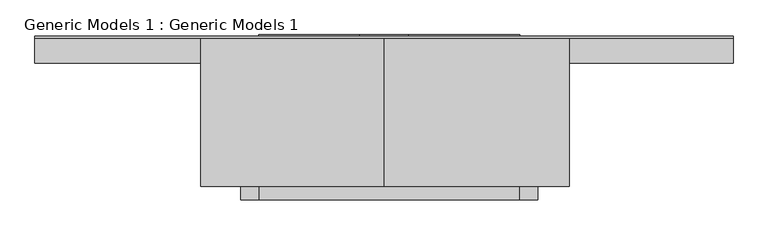
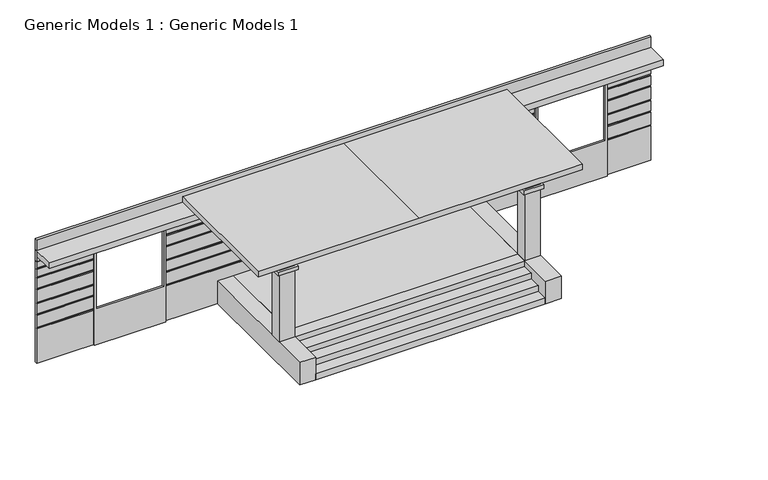
"""IFC4 building model written with IfcOpenShell, lengths in millimetres: proxy geometry, Generic Models 1 : Generic Models 1."""

from ifc_helpers import new_model, si_unit, frame, origin, origin_with_axes, place, context, project, spatial, polyline, outline, extrude, faceted_brep, source, transform, mapped, element, save


def generic_models_1_generic_models_1_130779d0(model_context):
    return source(origin(), model_context, "Body", "SolidModel", [
        extrude(outline(polyline([(2743.2, 5799.8347658), (2743.2, 3971.0347658), (0.0, 3971.0347658), (0.0, 5799.8347658), (2743.2, 5799.8347658)]), holes=[polyline([(2679.7, 5736.3347658), (977.9, 5736.3347658), (977.9, 4034.5347658), (2679.7, 4034.5347658), (2679.7, 5736.3347658)])]), frame((0.0, -1778.7594336, 0.0), z_axis=(0.0, 1.0, 0.0), x_axis=(0.0, 0.0, 1.0)), (0.0, 0.0, 1.0), 50.8),
        extrude(outline(polyline([(2743.2, -5477.7652342), (2743.2, -7306.5652342), (0.0, -7306.5652342), (0.0, -5477.7652342), (2743.2, -5477.7652342)]), holes=[polyline([(2679.7, -5541.2652342), (977.9, -5541.2652342), (977.9, -7243.0652342), (2679.7, -7243.0652342), (2679.7, -5541.2652342)])]), frame((0.0, -1778.7594336, 0.0), z_axis=(0.0, 1.0, 0.0), x_axis=(0.0, 0.0, 1.0)), (0.0, 0.0, 1.0), 50.8),
        extrude(outline(polyline([(-4131.5652342, -4452.9371224), (-4131.5652342, -4148.1371224), (-3725.1652342, -4148.1371224), (-3725.1652342, -4452.9371224), (-4131.5652342, -4452.9371224)])), frame((0.0, 0.0, 2540.0), z_axis=(0.0, 0.0, 1.0), x_axis=(1.0, 0.0, 0.0)), (0.0, 0.0, 1.0), 508.0),
        extrude(outline(polyline([(2142.2347658, -4452.9371224), (2142.2347658, -4148.1371224), (2548.6347658, -4148.1371224), (2548.6347658, -4452.9371224), (2142.2347658, -4452.9371224)])), frame((0.0, 0.0, 2540.0), z_axis=(0.0, 0.0, 1.0), x_axis=(1.0, 0.0, 0.0)), (0.0, 0.0, 1.0), 508.0),
        extrude(outline(polyline([(2599.4347658, -4503.7371224), (2091.4347658, -4503.7371224), (2091.4347658, -4097.3371224), (2599.4347658, -4097.3371224), (2599.4347658, -4503.7371224)])), frame((0.0, 0.0, 2438.4), z_axis=(0.0, 0.0, 1.0), x_axis=(1.0, 0.0, 0.0)), (0.0, 0.0, 1.0), 101.6),
        extrude(outline(polyline([(-3674.3652342, -4503.7371224), (-4182.3652342, -4503.7371224), (-4182.3652342, -4097.3371224), (-3674.3652342, -4097.3371224), (-3674.3652342, -4503.7371224)])), frame((0.0, 0.0, 2438.4), z_axis=(0.0, 0.0, 1.0), x_axis=(1.0, 0.0, 0.0)), (0.0, 0.0, 1.0), 101.6),
        extrude(outline(polyline([(2548.6347658, -4452.9371224), (2142.2347658, -4452.9371224), (2142.2347658, -4148.1371224), (2548.6347658, -4148.1371224), (2548.6347658, -4452.9371224)])), frame((0.0, 0.0, 609.6), z_axis=(0.0, 0.0, 1.0), x_axis=(1.0, 0.0, 0.0)), (0.0, 0.0, 1.0), 1828.8),
        extrude(outline(polyline([(-4131.5652342, -4148.1371224), (-3725.1652342, -4148.1371224), (-3725.1652342, -4452.9371224), (-4131.5652342, -4452.9371224), (-4131.5652342, -4148.1371224)])), frame((0.0, 0.0, 609.6), z_axis=(0.0, 0.0, 1.0), x_axis=(1.0, 0.0, 0.0)), (0.0, 0.0, 1.0), 1828.8),
        extrude(outline(polyline([(3048.0, -905.7652342), (3048.0, 3259.8347658), (3200.4, 3259.8347658), (3200.4, -905.7652342), (3200.4, -5020.5652342), (3048.0, -5020.5652342), (3048.0, -905.7652342)])), frame((0.0, -5062.5371224, 0.0), z_axis=(0.0, 1.0, 0.0), x_axis=(0.0, 0.0, 1.0)), (0.0, 0.0, 1.0), 3334.5776888),
        extrude(outline(polyline([(6942.8347658, -1727.9594336), (-8754.3652342, -1727.9594336), (-8754.3652342, -1677.1594336), (6942.8347658, -1677.1594336), (6942.8347658, -1727.9594336)])), frame((0.0, 0.0, 2743.2), z_axis=(0.0, 0.0, 1.0), x_axis=(1.0, 0.0, 0.0)), (0.0, 0.0, 1.0), 595.6731526),
        faceted_brep([(-8754.3652342, -1727.9594336, 0.0), (-4131.5652342, -1727.9594336, 0.0), (-4131.5652342, -1727.9594336, 600.1351718), (-1464.5652342, -1727.9594336, 600.1351718), (-1464.5652342, -1727.9594336, 2743.2), (-1997.9652342, -1727.9594336, 2743.2), (-1997.9652342, -1727.9594336, 1066.8), (-3521.9652342, -1727.9594336, 1066.8), (-3521.9652342, -1727.9594336, 1295.4), (-5477.7652342, -1727.9594336, 1295.4), (-5477.7652342, -1727.9594336, 969.0865476), (-3211.4976527, -1727.9594336, 969.0865476), (-1489.9652342, -1727.9594336, 969.0865476), (-1489.9652342, -1727.9594336, 926.1227307), (-3217.0111175, -1727.9594336, 926.1227307), (-5477.7652342, -1727.9594336, 926.1227307), (-5477.7652342, -1727.9594336, 914.4), (-7306.5652342, -1727.9594336, 914.4), (-7306.5652342, -1727.9594336, 926.1227307), (-8754.3652342, -1727.9594336, 926.1227307), (-1972.5652342, -1727.9594336, 1338.363817), (-1489.9652342, -1727.9594336, 1338.363817), (-1489.9652342, -1727.9594336, 1295.4), (-1972.5652342, -1727.9594336, 1295.4), (-1972.5652342, -1727.9594336, 1643.163817), (-1489.9652342, -1727.9594336, 1643.163817), (-1489.9652342, -1727.9594336, 1600.2), (-1972.5652342, -1727.9594336, 1600.2), (-1972.5652342, -1727.9594336, 2024.163817), (-1489.9652342, -1727.9594336, 2024.163817), (-1489.9652342, -1727.9594336, 1981.2), (-1972.5652342, -1727.9594336, 1981.2), (-1972.5652342, -1727.9594336, 2328.963817), (-1489.9652342, -1727.9594336, 2328.963817), (-1489.9652342, -1727.9594336, 2286.0), (-1972.5652342, -1727.9594336, 2286.0), (-1972.5652342, -1727.9594336, 2582.963817), (-1489.9652342, -1727.9594336, 2582.963817), (-1489.9652342, -1727.9594336, 2540.0), (-1972.5652342, -1727.9594336, 2540.0), (-3521.9652342, -1727.9594336, 2743.2), (-5477.7652342, -1727.9594336, 2743.2), (-5477.7652342, -1727.9594336, 2582.963817), (-3521.9652342, -1727.9594336, 2582.963817), (-7306.5652342, -1727.9594336, 2743.2), (-8754.3652342, -1727.9594336, 2743.2), (-8754.3652342, -1727.9594336, 2582.963817), (-7306.5652342, -1727.9594336, 2582.963817), (-8754.3652342, -1727.9594336, 1295.4), (-8754.3652342, -1727.9594336, 969.0865476), (-7306.5652342, -1727.9594336, 969.0865476), (-7306.5652342, -1727.9594336, 1295.4), (-8754.3652342, -1727.9594336, 1600.2), (-8754.3652342, -1727.9594336, 1338.363817), (-7306.5652342, -1727.9594336, 1338.363817), (-7306.5652342, -1727.9594336, 1600.2), (-8754.3652342, -1727.9594336, 1981.2), (-8754.3652342, -1727.9594336, 1643.163817), (-7306.5652342, -1727.9594336, 1643.163817), (-7306.5652342, -1727.9594336, 1981.2), (-8754.3652342, -1727.9594336, 2286.0), (-8754.3652342, -1727.9594336, 2024.163817), (-7306.5652342, -1727.9594336, 2024.163817), (-7306.5652342, -1727.9594336, 2286.0), (-8754.3652342, -1727.9594336, 2540.0), (-8754.3652342, -1727.9594336, 2328.963817), (-7306.5652342, -1727.9594336, 2328.963817), (-7306.5652342, -1727.9594336, 2540.0), (-3521.9652342, -1727.9594336, 1338.363817), (-3521.9652342, -1727.9594336, 1600.2), (-5477.7652342, -1727.9594336, 1600.2), (-5477.7652342, -1727.9594336, 1338.363817), (-3521.9652342, -1727.9594336, 1643.163817), (-3521.9652342, -1727.9594336, 1981.2), (-5477.7652342, -1727.9594336, 1981.2), (-5477.7652342, -1727.9594336, 1643.163817), (-3521.9652342, -1727.9594336, 2024.163817), (-3521.9652342, -1727.9594336, 2286.0), (-5477.7652342, -1727.9594336, 2286.0), (-5477.7652342, -1727.9594336, 2024.163817), (-3521.9652342, -1727.9594336, 2328.963817), (-3521.9652342, -1727.9594336, 2540.0), (-5477.7652342, -1727.9594336, 2540.0), (-5477.7652342, -1727.9594336, 2328.963817), (-4131.5652342, -1677.1594336, 600.1351718), (-4131.5652342, -1677.1594336, 0.0), (-8754.3652342, -1677.1594336, 0.0), (-8754.3652342, -1677.1594336, 2743.2), (-7306.5652342, -1677.1594336, 2743.2), (-7306.5652342, -1677.1594336, 914.4), (-5477.7652342, -1677.1594336, 914.4), (-5477.7652342, -1677.1594336, 2743.2), (-3521.9652342, -1677.1594336, 2743.2), (-3521.9652342, -1677.1594336, 1066.8), (-1997.9652342, -1677.1594336, 1066.8), (-1997.9652342, -1677.1594336, 2743.2), (-1464.5652342, -1677.1594336, 2743.2), (-1464.5652342, -1677.1594336, 600.1351718), (-8754.3652342, -1702.5594336, 926.1227307), (-8754.3652342, -1702.5594336, 969.0865476), (-8754.3652342, -1702.5594336, 1295.4), (-8754.3652342, -1702.5594336, 1338.363817), (-8754.3652342, -1702.5594336, 1600.2), (-8754.3652342, -1702.5594336, 1643.163817), (-8754.3652342, -1702.5594336, 1981.2), (-8754.3652342, -1702.5594336, 2024.163817), (-8754.3652342, -1702.5594336, 2286.0), (-8754.3652342, -1702.5594336, 2328.963817), (-8754.3652342, -1702.5594336, 2540.0), (-8754.3652342, -1702.5594336, 2582.963817), (-5477.7652342, -1702.5594336, 926.1227307), (-5477.7652342, -1702.5594336, 969.0865476), (-5477.7652342, -1702.5594336, 1295.4), (-5477.7652342, -1702.5594336, 1338.363817), (-5477.7652342, -1702.5594336, 1600.2), (-5477.7652342, -1702.5594336, 1643.163817), (-5477.7652342, -1702.5594336, 1981.2), (-5477.7652342, -1702.5594336, 2024.163817), (-5477.7652342, -1702.5594336, 2286.0), (-5477.7652342, -1702.5594336, 2328.963817), (-5477.7652342, -1702.5594336, 2540.0), (-5477.7652342, -1702.5594336, 2582.963817), (-7306.5652342, -1702.5594336, 2582.963817), (-7306.5652342, -1702.5594336, 2540.0), (-7306.5652342, -1702.5594336, 2328.963817), (-7306.5652342, -1702.5594336, 2286.0), (-7306.5652342, -1702.5594336, 2024.163817), (-7306.5652342, -1702.5594336, 1981.2), (-7306.5652342, -1702.5594336, 1643.163817), (-7306.5652342, -1702.5594336, 1600.2), (-7306.5652342, -1702.5594336, 1338.363817), (-7306.5652342, -1702.5594336, 1295.4), (-7306.5652342, -1702.5594336, 969.0865476), (-7306.5652342, -1702.5594336, 926.1227307), (-3521.9652342, -1702.5594336, 2582.963817), (-3521.9652342, -1702.5594336, 2540.0), (-3521.9652342, -1702.5594336, 2328.963817), (-3521.9652342, -1702.5594336, 2286.0), (-3521.9652342, -1702.5594336, 2024.163817), (-3521.9652342, -1702.5594336, 1981.2), (-3521.9652342, -1702.5594336, 1643.163817), (-3521.9652342, -1702.5594336, 1600.2), (-3521.9652342, -1702.5594336, 1338.363817), (-3521.9652342, -1702.5594336, 1295.4), (-3217.0111175, -1702.5594336, 926.1227307), (-1489.9652342, -1702.5594336, 926.1227307), (-1489.9652342, -1702.5594336, 969.0865476), (-3211.4976527, -1702.5594336, 969.0865476), (-1972.5652342, -1702.5594336, 1338.363817), (-1972.5652342, -1702.5594336, 1295.4), (-1489.9652342, -1702.5594336, 1295.4), (-1489.9652342, -1702.5594336, 1338.363817), (-1972.5652342, -1702.5594336, 1643.163817), (-1972.5652342, -1702.5594336, 1600.2), (-1489.9652342, -1702.5594336, 1600.2), (-1489.9652342, -1702.5594336, 1643.163817), (-1972.5652342, -1702.5594336, 2024.163817), (-1972.5652342, -1702.5594336, 1981.2), (-1489.9652342, -1702.5594336, 1981.2), (-1489.9652342, -1702.5594336, 2024.163817), (-1972.5652342, -1702.5594336, 2328.963817), (-1972.5652342, -1702.5594336, 2286.0), (-1489.9652342, -1702.5594336, 2286.0), (-1489.9652342, -1702.5594336, 2328.963817), (-1972.5652342, -1702.5594336, 2582.963817), (-1972.5652342, -1702.5594336, 2540.0), (-1489.9652342, -1702.5594336, 2540.0), (-1489.9652342, -1702.5594336, 2582.963817)], [[[0, 1, 2, 3, 4, 5, 6, 7, 8, 9, 10, 11, 12, 13, 14, 15, 16, 17, 18, 19], [20, 21, 22, 23], [24, 25, 26, 27], [28, 29, 30, 31], [32, 33, 34, 35], [36, 37, 38, 39]], [[40, 41, 42, 43]], [[44, 45, 46, 47]], [[48, 49, 50, 51]], [[52, 53, 54, 55]], [[56, 57, 58, 59]], [[60, 61, 62, 63]], [[64, 65, 66, 67]], [[68, 69, 70, 71]], [[72, 73, 74, 75]], [[76, 77, 78, 79]], [[80, 81, 82, 83]], [[84, 85, 86, 87, 88, 89, 90, 91, 92, 93, 94, 95, 96, 97]], [[87, 45, 44, 88]], [[5, 4, 96, 95]], [[41, 40, 92, 91]], [[87, 86, 0, 19, 98, 99, 49, 48, 100, 101, 53, 52, 102, 103, 57, 56, 104, 105, 61, 60, 106, 107, 65, 64, 108, 109, 46, 45]], [[1, 0, 86, 85]], [[2, 1, 85, 84]], [[2, 84, 97, 3]], [[90, 16, 15, 110, 111, 10, 9, 112, 113, 71, 70, 114, 115, 75, 74, 116, 117, 79, 78, 118, 119, 83, 82, 120, 121, 42, 41, 91]], [[16, 90, 89, 17]], [[17, 89, 88, 44, 47, 122, 123, 67, 66, 124, 125, 63, 62, 126, 127, 59, 58, 128, 129, 55, 54, 130, 131, 51, 50, 132, 133, 18]], [[94, 6, 5, 95]], [[6, 94, 93, 7]], [[7, 93, 92, 40, 43, 134, 135, 81, 80, 136, 137, 77, 76, 138, 139, 73, 72, 140, 141, 69, 68, 142, 143, 8]], [[4, 3, 97, 96]], [[98, 133, 132, 99]], [[100, 131, 130, 101]], [[102, 129, 128, 103]], [[104, 127, 126, 105]], [[106, 125, 124, 107]], [[108, 123, 122, 109]], [[110, 144, 145, 146, 147, 111]], [[112, 143, 142, 113]], [[114, 141, 140, 115]], [[116, 139, 138, 117]], [[118, 137, 136, 119]], [[120, 135, 134, 121]], [[148, 149, 150, 151]], [[152, 153, 154, 155]], [[156, 157, 158, 159]], [[160, 161, 162, 163]], [[164, 165, 166, 167]], [[99, 132, 50, 49]], [[133, 98, 19, 18]], [[101, 130, 54, 53]], [[131, 100, 48, 51]], [[103, 128, 58, 57]], [[129, 102, 52, 55]], [[105, 126, 62, 61]], [[127, 104, 56, 59]], [[107, 124, 66, 65]], [[125, 106, 60, 63]], [[109, 122, 47, 46]], [[123, 108, 64, 67]], [[111, 147, 11, 10]], [[147, 146, 12, 11]], [[146, 145, 13, 12]], [[145, 144, 14, 13]], [[144, 110, 15, 14]], [[113, 142, 68, 71]], [[143, 112, 9, 8]], [[115, 140, 72, 75]], [[141, 114, 70, 69]], [[117, 138, 76, 79]], [[139, 116, 74, 73]], [[119, 136, 80, 83]], [[137, 118, 78, 77]], [[121, 134, 43, 42]], [[135, 120, 82, 81]], [[148, 151, 21, 20]], [[151, 150, 22, 21]], [[150, 149, 23, 22]], [[149, 148, 20, 23]], [[152, 155, 25, 24]], [[155, 154, 26, 25]], [[154, 153, 27, 26]], [[153, 152, 24, 27]], [[156, 159, 29, 28]], [[159, 158, 30, 29]], [[158, 157, 31, 30]], [[157, 156, 28, 31]], [[160, 163, 33, 32]], [[163, 162, 34, 33]], [[162, 161, 35, 34]], [[161, 160, 32, 35]], [[164, 167, 37, 36]], [[167, 166, 38, 37]], [[166, 165, 39, 38]], [[165, 164, 36, 39]]]),
        faceted_brep([(2548.6347658, -1727.9594336, 600.1351718), (2548.6347658, -1727.9594336, 0.0), (3971.0347658, -1727.9594336, 0.0), (6942.8347658, -1727.9594336, 0.0), (6942.8347658, -1727.9594336, 926.1227307), (5799.8347658, -1727.9594336, 926.1227307), (5799.8347658, -1727.9594336, 914.4), (3971.0347658, -1727.9594336, 914.4), (3971.0347658, -1727.9594336, 926.1227307), (1735.8347658, -1727.9594336, 926.1227307), (1735.8347658, -1727.9594336, 969.0865476), (3971.0347658, -1727.9594336, 969.0865476), (3971.0347658, -1727.9594336, 1295.4), (1735.8347658, -1727.9594336, 1295.4), (1735.8347658, -1727.9594336, 1066.8), (211.8347658, -1727.9594336, 1066.8), (211.8347658, -1727.9594336, 2743.2), (-346.9652342, -1727.9594336, 2743.2), (-346.9652342, -1727.9594336, 600.1351718), (199.1347658, -1727.9594336, 962.7365476), (199.1347658, -1727.9594336, 926.1227307), (-334.2652342, -1727.9594336, 926.1227307), (-334.2652342, -1727.9594336, 962.7365476), (199.1347658, -1727.9594336, 1338.363817), (199.1347658, -1727.9594336, 1295.4), (-334.2652342, -1727.9594336, 1295.4), (-334.2652342, -1727.9594336, 1338.363817), (199.1347658, -1727.9594336, 1643.163817), (199.1347658, -1727.9594336, 1600.2), (-334.2652342, -1727.9594336, 1600.2), (-334.2652342, -1727.9594336, 1643.163817), (199.1347658, -1727.9594336, 2024.163817), (199.1347658, -1727.9594336, 1981.2), (-334.2652342, -1727.9594336, 1981.2), (-334.2652342, -1727.9594336, 2024.163817), (199.1347658, -1727.9594336, 2328.963817), (199.1347658, -1727.9594336, 2286.0), (-334.2652342, -1727.9594336, 2286.0), (-334.2652342, -1727.9594336, 2328.963817), (199.1347658, -1727.9594336, 2582.963817), (199.1347658, -1727.9594336, 2540.0), (-334.2652342, -1727.9594336, 2540.0), (-334.2652342, -1727.9594336, 2582.963817), (6942.8347658, -1727.9594336, 2743.2), (5799.8347658, -1727.9594336, 2743.2), (5799.8347658, -1727.9594336, 2582.963817), (6942.8347658, -1727.9594336, 2582.963817), (3971.0347658, -1727.9594336, 2743.2), (1735.8347658, -1727.9594336, 2743.2), (1735.8347658, -1727.9594336, 2582.963817), (3971.0347658, -1727.9594336, 2582.963817), (6942.8347658, -1727.9594336, 962.7365476), (6942.8347658, -1727.9594336, 1295.4), (5799.8347658, -1727.9594336, 1295.4), (5799.8347658, -1727.9594336, 962.7365476), (6942.8347658, -1727.9594336, 1338.363817), (6942.8347658, -1727.9594336, 1600.2), (5799.8347658, -1727.9594336, 1600.2), (5799.8347658, -1727.9594336, 1338.363817), (6942.8347658, -1727.9594336, 1643.163817), (6942.8347658, -1727.9594336, 1981.2), (5799.8347658, -1727.9594336, 1981.2), (5799.8347658, -1727.9594336, 1643.163817), (6942.8347658, -1727.9594336, 2024.163817), (6942.8347658, -1727.9594336, 2286.0), (5799.8347658, -1727.9594336, 2286.0), (5799.8347658, -1727.9594336, 2024.163817), (6942.8347658, -1727.9594336, 2328.963817), (6942.8347658, -1727.9594336, 2540.0), (5799.8347658, -1727.9594336, 2540.0), (5799.8347658, -1727.9594336, 2328.963817), (3971.0347658, -1727.9594336, 1338.363817), (3971.0347658, -1727.9594336, 1600.2), (1735.8347658, -1727.9594336, 1600.2), (1735.8347658, -1727.9594336, 1338.363817), (3971.0347658, -1727.9594336, 1643.163817), (3971.0347658, -1727.9594336, 1981.2), (1735.8347658, -1727.9594336, 1981.2), (1735.8347658, -1727.9594336, 1643.163817), (3971.0347658, -1727.9594336, 2024.163817), (3971.0347658, -1727.9594336, 2286.0), (1735.8347658, -1727.9594336, 2286.0), (1735.8347658, -1727.9594336, 2024.163817), (3971.0347658, -1727.9594336, 2328.963817), (3971.0347658, -1727.9594336, 2540.0), (1735.8347658, -1727.9594336, 2540.0), (1735.8347658, -1727.9594336, 2328.963817), (6942.8347658, -1677.1594336, 2743.2), (6942.8347658, -1677.1594336, 0.0), (3971.0347658, -1677.1594336, 0.0), (2548.6347658, -1677.1594336, 0.0), (2548.6347658, -1677.1594336, 600.1351718), (-346.9652342, -1677.1594336, 600.1351718), (-346.9652342, -1677.1594336, 2743.2), (211.8347658, -1677.1594336, 2743.2), (211.8347658, -1677.1594336, 1066.8), (1735.8347658, -1677.1594336, 1066.8), (1735.8347658, -1677.1594336, 2743.2), (3971.0347658, -1677.1594336, 2743.2), (3971.0347658, -1677.1594336, 914.4), (5799.8347658, -1677.1594336, 914.4), (5799.8347658, -1677.1594336, 2743.2), (6942.8347658, -1702.5594336, 2582.963817), (6942.8347658, -1702.5594336, 2540.0), (6942.8347658, -1702.5594336, 2328.963817), (6942.8347658, -1702.5594336, 2286.0), (6942.8347658, -1702.5594336, 2024.163817), (6942.8347658, -1702.5594336, 1981.2), (6942.8347658, -1702.5594336, 1643.163817), (6942.8347658, -1702.5594336, 1600.2), (6942.8347658, -1702.5594336, 1338.363817), (6942.8347658, -1702.5594336, 1295.4), (6942.8347658, -1702.5594336, 962.7365476), (6942.8347658, -1702.5594336, 926.1227307), (1735.8347658, -1702.5594336, 1295.4), (1735.8347658, -1702.5594336, 1338.363817), (1735.8347658, -1702.5594336, 1600.2), (1735.8347658, -1702.5594336, 1643.163817), (1735.8347658, -1702.5594336, 1981.2), (1735.8347658, -1702.5594336, 2024.163817), (1735.8347658, -1702.5594336, 2286.0), (1735.8347658, -1702.5594336, 2328.963817), (1735.8347658, -1702.5594336, 2540.0), (1735.8347658, -1702.5594336, 2582.963817), (5799.8347658, -1702.5594336, 926.1227307), (5799.8347658, -1702.5594336, 962.7365476), (5799.8347658, -1702.5594336, 1295.4), (5799.8347658, -1702.5594336, 1338.363817), (5799.8347658, -1702.5594336, 1600.2), (5799.8347658, -1702.5594336, 1643.163817), (5799.8347658, -1702.5594336, 1981.2), (5799.8347658, -1702.5594336, 2024.163817), (5799.8347658, -1702.5594336, 2286.0), (5799.8347658, -1702.5594336, 2328.963817), (5799.8347658, -1702.5594336, 2540.0), (5799.8347658, -1702.5594336, 2582.963817), (3971.0347658, -1702.5594336, 2582.963817), (3971.0347658, -1702.5594336, 2540.0), (3971.0347658, -1702.5594336, 2328.963817), (3971.0347658, -1702.5594336, 2286.0), (3971.0347658, -1702.5594336, 2024.163817), (3971.0347658, -1702.5594336, 1981.2), (3971.0347658, -1702.5594336, 1643.163817), (3971.0347658, -1702.5594336, 1600.2), (3971.0347658, -1702.5594336, 1338.363817), (3971.0347658, -1702.5594336, 1295.4), (3971.0347658, -1702.5594336, 969.0865476), (3971.0347658, -1702.5594336, 926.1227307), (1735.8347658, -1702.5594336, 969.0865476), (1735.8347658, -1702.5594336, 926.1227307), (199.1347658, -1702.5594336, 962.7365476), (-334.2652342, -1702.5594336, 962.7365476), (-334.2652342, -1702.5594336, 926.1227307), (199.1347658, -1702.5594336, 926.1227307), (199.1347658, -1702.5594336, 1338.363817), (-334.2652342, -1702.5594336, 1338.363817), (-334.2652342, -1702.5594336, 1295.4), (199.1347658, -1702.5594336, 1295.4), (199.1347658, -1702.5594336, 1643.163817), (-334.2652342, -1702.5594336, 1643.163817), (-334.2652342, -1702.5594336, 1600.2), (199.1347658, -1702.5594336, 1600.2), (199.1347658, -1702.5594336, 2024.163817), (-334.2652342, -1702.5594336, 2024.163817), (-334.2652342, -1702.5594336, 1981.2), (199.1347658, -1702.5594336, 1981.2), (199.1347658, -1702.5594336, 2328.963817), (-334.2652342, -1702.5594336, 2328.963817), (-334.2652342, -1702.5594336, 2286.0), (199.1347658, -1702.5594336, 2286.0), (199.1347658, -1702.5594336, 2582.963817), (-334.2652342, -1702.5594336, 2582.963817), (-334.2652342, -1702.5594336, 2540.0), (199.1347658, -1702.5594336, 2540.0)], [[[0, 1, 2, 3, 4, 5, 6, 7, 8, 9, 10, 11, 12, 13, 14, 15, 16, 17, 18], [19, 20, 21, 22], [23, 24, 25, 26], [27, 28, 29, 30], [31, 32, 33, 34], [35, 36, 37, 38], [39, 40, 41, 42]], [[43, 44, 45, 46]], [[47, 48, 49, 50]], [[51, 52, 53, 54]], [[55, 56, 57, 58]], [[59, 60, 61, 62]], [[63, 64, 65, 66]], [[67, 68, 69, 70]], [[71, 72, 73, 74]], [[75, 76, 77, 78]], [[79, 80, 81, 82]], [[83, 84, 85, 86]], [[87, 88, 89, 90, 91, 92, 93, 94, 95, 96, 97, 98, 99, 100, 101]], [[43, 87, 101, 44]], [[48, 47, 98, 97]], [[17, 16, 94, 93]], [[91, 0, 18, 92]], [[1, 0, 91, 90]], [[2, 1, 90, 89]], [[3, 2, 89, 88]], [[88, 87, 43, 46, 102, 103, 68, 67, 104, 105, 64, 63, 106, 107, 60, 59, 108, 109, 56, 55, 110, 111, 52, 51, 112, 113, 4, 3]], [[18, 17, 93, 92]], [[96, 14, 13, 114, 115, 74, 73, 116, 117, 78, 77, 118, 119, 82, 81, 120, 121, 86, 85, 122, 123, 49, 48, 97]], [[14, 96, 95, 15]], [[15, 95, 94, 16]], [[100, 6, 5, 124, 125, 54, 53, 126, 127, 58, 57, 128, 129, 62, 61, 130, 131, 66, 65, 132, 133, 70, 69, 134, 135, 45, 44, 101]], [[6, 100, 99, 7]], [[7, 99, 98, 47, 50, 136, 137, 84, 83, 138, 139, 80, 79, 140, 141, 76, 75, 142, 143, 72, 71, 144, 145, 12, 11, 146, 147, 8]], [[148, 149, 147, 146]], [[112, 125, 124, 113]], [[114, 145, 144, 115]], [[110, 127, 126, 111]], [[116, 143, 142, 117]], [[108, 129, 128, 109]], [[118, 141, 140, 119]], [[106, 131, 130, 107]], [[120, 139, 138, 121]], [[104, 133, 132, 105]], [[122, 137, 136, 123]], [[102, 135, 134, 103]], [[150, 151, 152, 153]], [[154, 155, 156, 157]], [[158, 159, 160, 161]], [[162, 163, 164, 165]], [[166, 167, 168, 169]], [[170, 171, 172, 173]], [[148, 146, 11, 10]], [[147, 149, 9, 8]], [[149, 148, 10, 9]], [[113, 124, 5, 4]], [[125, 112, 51, 54]], [[115, 144, 71, 74]], [[145, 114, 13, 12]], [[111, 126, 53, 52]], [[127, 110, 55, 58]], [[117, 142, 75, 78]], [[143, 116, 73, 72]], [[109, 128, 57, 56]], [[129, 108, 59, 62]], [[119, 140, 79, 82]], [[141, 118, 77, 76]], [[107, 130, 61, 60]], [[131, 106, 63, 66]], [[121, 138, 83, 86]], [[139, 120, 81, 80]], [[105, 132, 65, 64]], [[133, 104, 67, 70]], [[123, 136, 50, 49]], [[137, 122, 85, 84]], [[103, 134, 69, 68]], [[135, 102, 46, 45]], [[150, 153, 20, 19]], [[153, 152, 21, 20]], [[152, 151, 22, 21]], [[151, 150, 19, 22]], [[154, 157, 24, 23]], [[157, 156, 25, 24]], [[156, 155, 26, 25]], [[155, 154, 23, 26]], [[158, 161, 28, 27]], [[161, 160, 29, 28]], [[160, 159, 30, 29]], [[159, 158, 27, 30]], [[162, 165, 32, 31]], [[165, 164, 33, 32]], [[164, 163, 34, 33]], [[163, 162, 31, 34]], [[166, 169, 36, 35]], [[169, 168, 37, 36]], [[168, 167, 38, 37]], [[167, 166, 35, 38]], [[170, 173, 40, 39]], [[173, 172, 41, 40]], [[172, 171, 42, 41]], [[171, 170, 39, 42]]]),
        extrude(outline(polyline([(6942.8347658, -2286.7594336), (2548.6347658, -2286.7594336), (2548.6347658, -1677.1594336), (6942.8347658, -1677.1594336), (6942.8347658, -2286.7594336)])), frame((0.0, 0.0, 2895.6), z_axis=(0.0, 0.0, 1.0), x_axis=(1.0, 0.0, 0.0)), (0.0, 0.0, 1.0), 152.4),
        extrude(outline(polyline([(-4131.5652342, -2286.7594336), (-8754.3652342, -2286.7594336), (-8754.3652342, -1677.1594336), (-4131.5652342, -1677.1594336), (-4131.5652342, -2286.7594336)])), frame((0.0, 0.0, 2895.6), z_axis=(0.0, 0.0, 1.0), x_axis=(1.0, 0.0, 0.0)), (0.0, 0.0, 1.0), 152.4),
        faceted_brep([(2142.2347658, -4148.1371224, 0.0), (2142.2347658, -1652.0198001, 0.0), (2142.2347658, -1652.0198001, 609.6), (2142.2347658, -4148.1371224, 609.6), (-3725.1652342, -4148.1371224, 0.0), (-3725.1652342, -4148.1371224, 609.6), (-3725.1652342, -1652.0198001, 609.6), (-3725.1652342, -1652.0198001, 0.0), (-1464.5652342, -1652.0198001, 609.6), (-1464.5652342, -1652.0198001, 584.2), (-346.9652342, -1652.0198001, 584.2), (-346.9652342, -1652.0198001, 609.6), (-346.9652342, -1727.9594336, 609.6), (-1464.5652342, -1727.9594336, 609.6), (-346.9652342, -1727.9594336, 584.2), (-1464.5652342, -1727.9594336, 584.2)], [[[0, 1, 2, 3]], [[4, 5, 6, 7]], [[1, 0, 4, 7]], [[2, 1, 7, 6, 8, 9, 10, 11]], [[3, 2, 11, 12, 13, 8, 6, 5]], [[0, 3, 5, 4]], [[14, 15, 13, 12]], [[14, 12, 11, 10]], [[15, 14, 10, 9]], [[13, 15, 9, 8]]]),
        extrude(outline(polyline([(2548.6347658, -5367.3371224), (2142.2347658, -5367.3371224), (2142.2347658, -1677.1594336), (2548.6347658, -1677.1594336), (2548.6347658, -5367.3371224)])), origin_with_axes(), (0.0, 0.0, 1.0), 609.6),
        extrude(outline(polyline([(-3725.1652342, -5367.3371224), (-4131.5652342, -5367.3371224), (-4131.5652342, -1677.1594336), (-3725.1652342, -1677.1594336), (-3725.1652342, -5367.3371224)])), origin_with_axes(), (0.0, 0.0, 1.0), 609.6),
        extrude(outline(polyline([(-4148.1371224, 609.6), (-4148.1371224, 0.0), (-5367.3371224, 0.0), (-5367.3371224, 152.4), (-5062.5371224, 152.4), (-5062.5371224, 304.8), (-4757.7371224, 304.8), (-4757.7371224, 457.2), (-4452.9371224, 457.2), (-4452.9371224, 609.6), (-4148.1371224, 609.6)])), frame((-3725.1652342, 0.0, 0.0), z_axis=(1.0, 0.0, 0.0), x_axis=(0.0, 1.0, 0.0)), (0.0, 0.0, 1.0), 5867.4),
    ])


if __name__ == "__main__":
    model = new_model("IFC4")
    model_context = context("Model", 3, world=origin())
    ifc_project = project(units=[si_unit("LENGTHUNIT", "METRE", prefix="MILLI")], contexts=[model_context])
    site = spatial("IfcSite", under=ifc_project)
    building = spatial("IfcBuilding", under=site)
    placement = place(None, origin())
    generic_models_1_generic_models_1_shape = generic_models_1_generic_models_1_130779d0(model_context)
    element("IfcBuildingElementProxy", 1, Name="Generic Models 1 : Generic Models 1", ObjectType="Generic Models 1 : Generic Models 1", at=placement, inside=building, context=model_context, shape_type="MappedRepresentation", body=[
        mapped(generic_models_1_generic_models_1_shape, transform((0.0, 0.0, 0.0), x_axis=(1.0, 0.0, 0.0), y_axis=(0.0, 1.0, 0.0), z_axis=(0.0, 0.0, 1.0))),
    ])
    save(model, "model.ifc")

# Revit data of these elements
# Element 1 (IfcBuildingElementProxy, "Generic Models 1 : Generic Models 1")
#   Materials on its faces: "Gypsum Wall Board", "rock b"
# Materials
#   "Gypsum Wall Board": class "Generic", colour RGB 127 127 127, transparency 0, Description = "Gypsum Wall Board", Cost = 0
#   "rock b": class "Generic", colour RGB 120 120 120, transparency 0, Cost = 0
